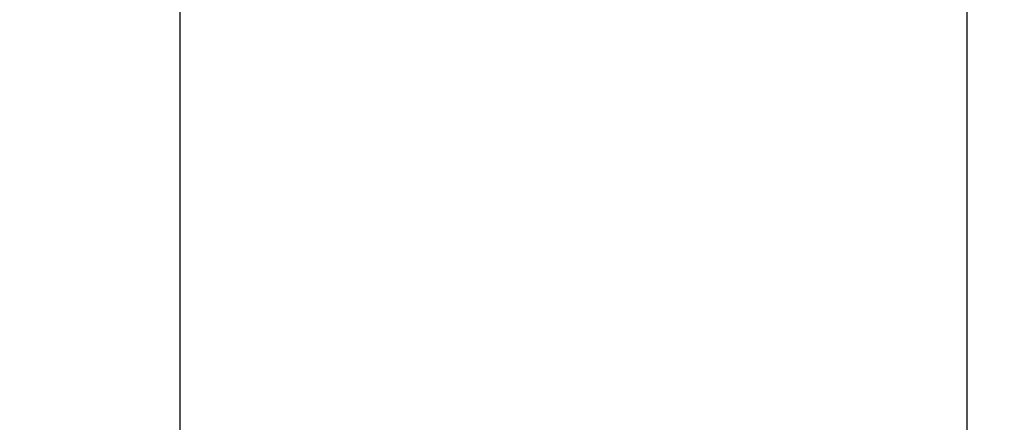
# Model space of a CAD drawing. Units: inches. Extents: x 2091 to 2899, y 967 to 2217.
# Tile 20 of 256: x 2351 to 2390, y 1064 to 1080. Entities that reach past the tile are written whole.
import ezdxf

# ---------------------------------------------------------------- set-up
doc = ezdxf.new("R2010")
doc.units = ezdxf.units.IN
doc.layers.add('A-ANNO-DIMS', color=2, linetype='Continuous', lineweight=18)
doc.styles.get("Standard").update_dxf_attribs({"font": 'arial.ttf'})
doc.dimstyles.new('ISO-25', dxfattribs={"dimtxt": 4, "dimasz": 4, "dimexe": 1.25, "dimexo": 0.625, "dimtad": 1, "dimdec": 0, "dimlunit": 3, "dimtxsty": 'Standard', "dimcen": 2.5, "dimadec": 0, "dimazin": 0, "dimtfac": 1, "dimtdec": 0, "dimtmove": 0, "dimatfit": 3, "dimfxl": 1, "dimarcsym": 0})

# ---------------------------------------------------------------- blocks, each defined once
blk = doc.blocks.new('*D68')
at = {"layer": 'A-ANNO-DIMS', "color": 0, "lineweight": -2, "transparency": 16777216}
for p, q in [((2317.144, 1535.794), (2317.144, 969.464)), ((2459.384, 1535.794), (2459.384, 969.464)), ((2321.144, 970.714), (2455.384, 970.714))]:
    blk.add_line(p, q, dxfattribs=at)
at = {"layer": 'A-ANNO-DIMS', "color": 0, "transparency": 16777216}
for points in [[(2321.144, 971.381), (2321.144, 970.048), (2317.144, 970.714)], [(2455.384, 971.381), (2455.384, 970.048), (2459.384, 970.714)]]:
    blk.add_solid(points, dxfattribs=at)
at = {"layer": 'Defpoints', "color": 0, "transparency": 16777216}
for p in [(2317.144, 1536.419), (2459.384, 1536.419), (2459.384, 970.714)]:
    blk.add_point(p, dxfattribs=at)
at = {"layer": 'A-ANNO-DIMS', "color": 0, "transparency": 16777216, "insert": (2388.264, 973.382), "char_height": 4, "attachment_point": 5}
blk.add_mtext('11\'-10"', dxfattribs=at)
blk = doc.blocks.new('*D71')
at = {"layer": 'A-ANNO-DIMS', "color": 0, "lineweight": -2, "transparency": 16777216}
for p, q in [((2212.144, 1351.294), (2212.144, 969.464)), ((2452.144, 1351.294), (2452.144, 969.464)), ((2216.144, 970.714), (2448.144, 970.714))]:
    blk.add_line(p, q, dxfattribs=at)
at = {"layer": 'A-ANNO-DIMS', "color": 0, "transparency": 16777216}
for points in [[(2216.144, 971.381), (2216.144, 970.048), (2212.144, 970.714)], [(2448.144, 971.381), (2448.144, 970.048), (2452.144, 970.714)]]:
    blk.add_solid(points, dxfattribs=at)
at = {"layer": 'Defpoints', "color": 0, "transparency": 16777216}
for p in [(2212.144, 1351.919), (2452.144, 1351.919), (2452.144, 970.714)]:
    blk.add_point(p, dxfattribs=at)
at = {"layer": 'A-ANNO-DIMS', "color": 0, "transparency": 16777216, "insert": (2332.144, 973.382), "char_height": 4, "attachment_point": 5}
blk.add_mtext('20\'-0"', dxfattribs=at)
blk = doc.blocks.new('*D82')
at = {"layer": 'A-ANNO-DIMS', "color": 0, "lineweight": -2, "transparency": 16777216}
for p, q in [((2357.434, 1549.361), (2357.434, 969.464)), ((2388.969, 1549.361), (2388.969, 969.464)), ((2361.434, 970.714), (2384.969, 970.714))]:
    blk.add_line(p, q, dxfattribs=at)
at = {"layer": 'A-ANNO-DIMS', "color": 0, "transparency": 16777216}
for points in [[(2361.434, 971.381), (2361.434, 970.048), (2357.434, 970.714)], [(2384.969, 971.381), (2384.969, 970.048), (2388.969, 970.714)]]:
    blk.add_solid(points, dxfattribs=at)
at = {"layer": 'Defpoints', "color": 0, "transparency": 16777216}
for p in [(2357.434, 1549.986), (2388.969, 1549.986), (2388.969, 970.714)]:
    blk.add_point(p, dxfattribs=at)
at = {"layer": 'A-ANNO-DIMS', "color": 0, "transparency": 16777216, "insert": (2373.202, 973.408), "char_height": 4, "attachment_point": 5}
blk.add_mtext('2\'-7 1/2"', dxfattribs=at)

msp = doc.modelspace()

# ---------------------------------------------------------------- dimensions: what is measured, and where the dimension line sits
at = {"layer": 'A-ANNO-DIMS'}
for base, p1, p2, picture, middle in [((2388.969, 970.714), (2357.434, 1549.986), (2388.969, 1549.986), '*D82', (2373.202, 973.408)), ((2459.384, 970.714), (2317.144, 1536.419), (2459.384, 1536.419), '*D68', (2388.264, 973.382)), ((2452.144, 970.714), (2212.144, 1351.919), (2452.144, 1351.919), '*D71', (2332.144, 973.382))]:
    dim = msp.add_linear_dim(base=base, p1=p1, p2=p2, dimstyle='ISO-25', override={"dimdec": 1, "dimlfac": 1, "dimrnd": 0, "dimzin": 1, "dimdsep": 46, "dimlunit": 4, "dimfrac": 2}, dxfattribs=at)
    dim.commit()
    dim.dimension.update_dxf_attribs({"geometry": picture, "text_midpoint": middle})

doc.saveas('drawing.dxf')
